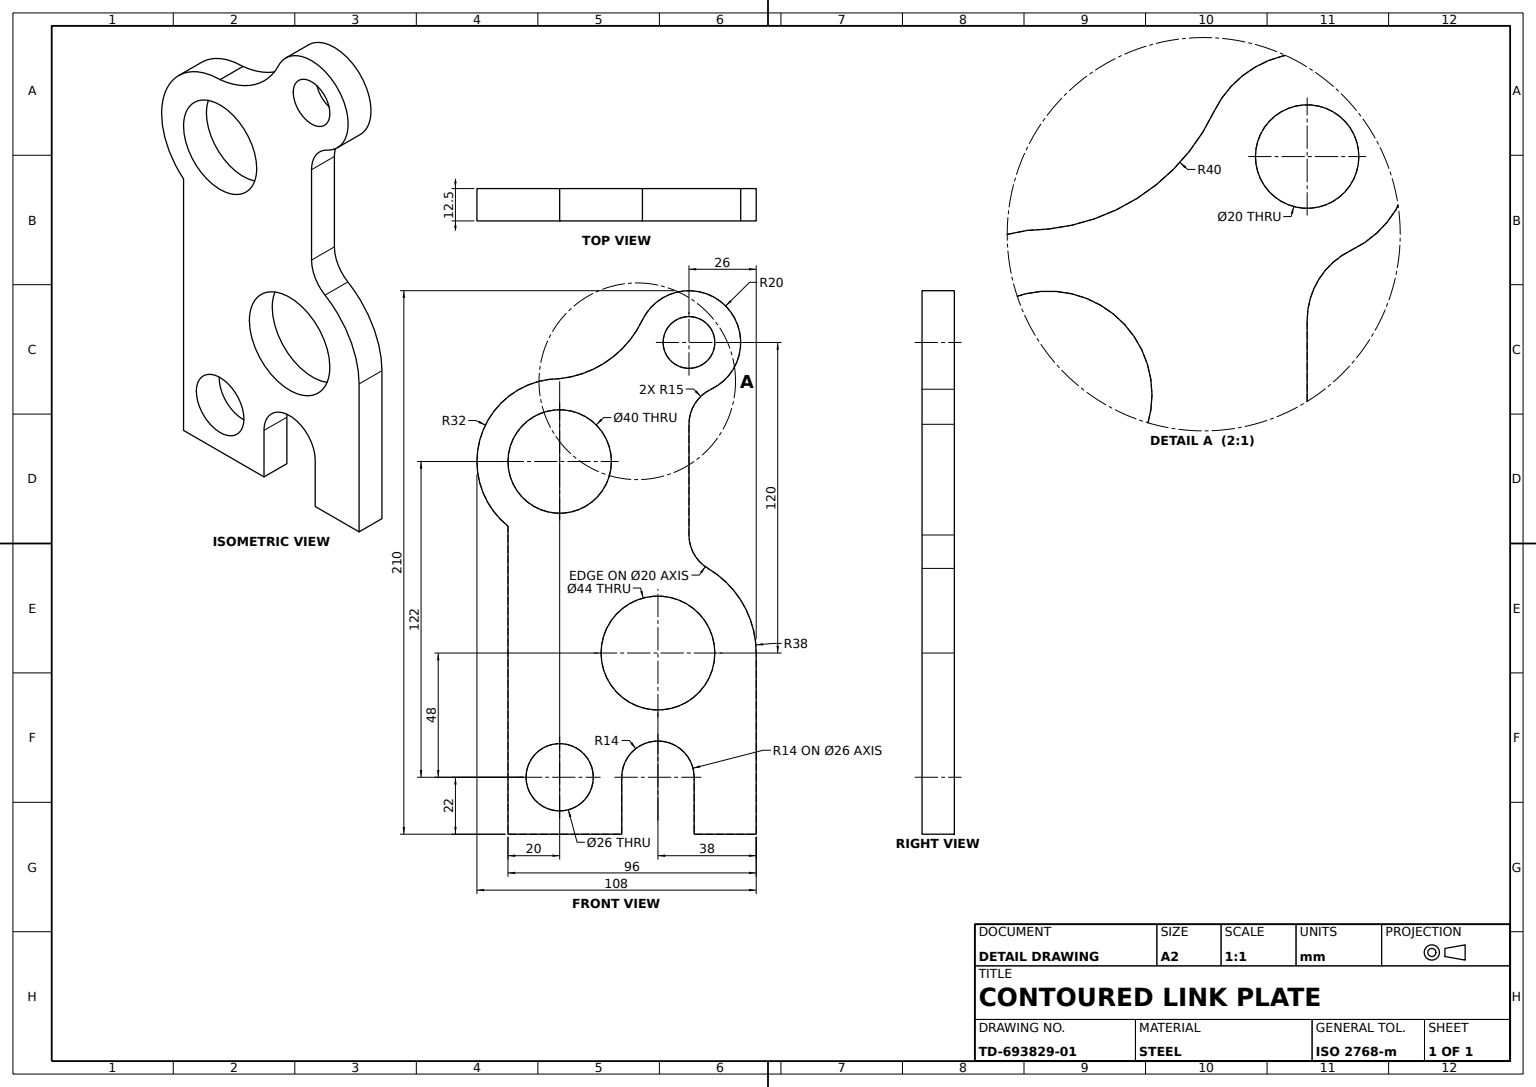
SolidWorks part; units mm, degrees
material "Plain Carbon Steel"
ref_plane "Front Plane" through (0, 0, 0) normal (0, 0, 1) x (1, 0, 0)
ref_plane "Top Plane" through (0, 0, 0) normal (0, 1, 0) x (1, 0, 0)
ref_plane "Right Plane" through (0, 0, 0) normal (1, 0, 0) x (0, 0, -1)
sketch "Bracket Profile Sketch" plane through (0, 0, 0) normal (0, 0, 1) x (1, 0, 0)
  line L0 (0, 0) -> (44, 0)
  line L1 (96, 0) -> (96, 70)
  line L2 (58, 70) -> (58, 43) construction
  line L3 (58, 22) -> (20, 22) construction
  line L4 (72, 0) -> (96, 0)
  line L5 (0, 0) -> (0, 119.02)
  line L6 (58, 0) -> (58, 36) construction
  line L7 (44, 22) -> (44, 0)
  line L8 (72, 22) -> (72, 0)
  line L9 (58, 70) -> (96, 70) construction
  line L10 (96, 70) -> (96, 43) construction
  line L11 (20, 22) -> (20, 144) construction
  line L12 (58, 36) -> (58, 22) construction
  line L13 (58, 43) -> (58, 70) construction
  line L14 (96, 43) -> (96, 70)
  line L15 (70, 190) -> (70, 115.607)
  line L16 (20, 22) -> (20, 0) construction
  line L17 (58, 70) -> (58, 108) construction
  line L18 (58, 70) -> (96, 70) construction
  line L19 (58, 43) -> (96, 43)
  line L20 (31.2605, 43) -> (58, 43)
  circle A0 centre (20, 144) radius 32
  circle A1 centre (20, 144) radius 20
  circle A3 centre (58, 70) radius 22
  circle A4 centre (20, 22) radius 13
  arc A5 (72, 22) -> (44, 22) centre (58, 22) ccw
  circle A6 centre (70, 190) radius 20
  circle A9 centre (70, 190) radius 10
  arc A12 (70, 115.607) -> (77.3585, 102.6994) centre (85, 115.607) ccw
  arc A13 (84.7395, 43) -> (31.2605, 43) centre (58, 70) ccw
  arc A14 (52, 198.7178) -> (20, 176) centre (15.8221, 215.7812) cw
  dimension "D4" = 64
  dimension "D5" = 40
  dimension "D2" = 50
  dimension "D3" = 44
  dimension "D7" = 70
  dimension "D6" = 26
  dimension "D10" = 27
  dimension "D11" = 120
  dimension "D12" = 40
  dimension "D13" = 20
  dimension "D14" = 14
  dimension "D17" = 38
  dimension "D18" = 40
  dimension "D19" = 15
  dimension "D1" = 96
  dimension "D8" = 48
  dimension "D9" = 122
  dimension "D15" = 38
  dimension "D16" = 38
  dimension "D20" = 18
extrude "Bracket Plate 12.5mm" add sketch "Bracket Profile Sketch" along normal blind 12.5
fillet "Edge Fillet R15" radius 15 1 edges at (70, 170, 6.25)
